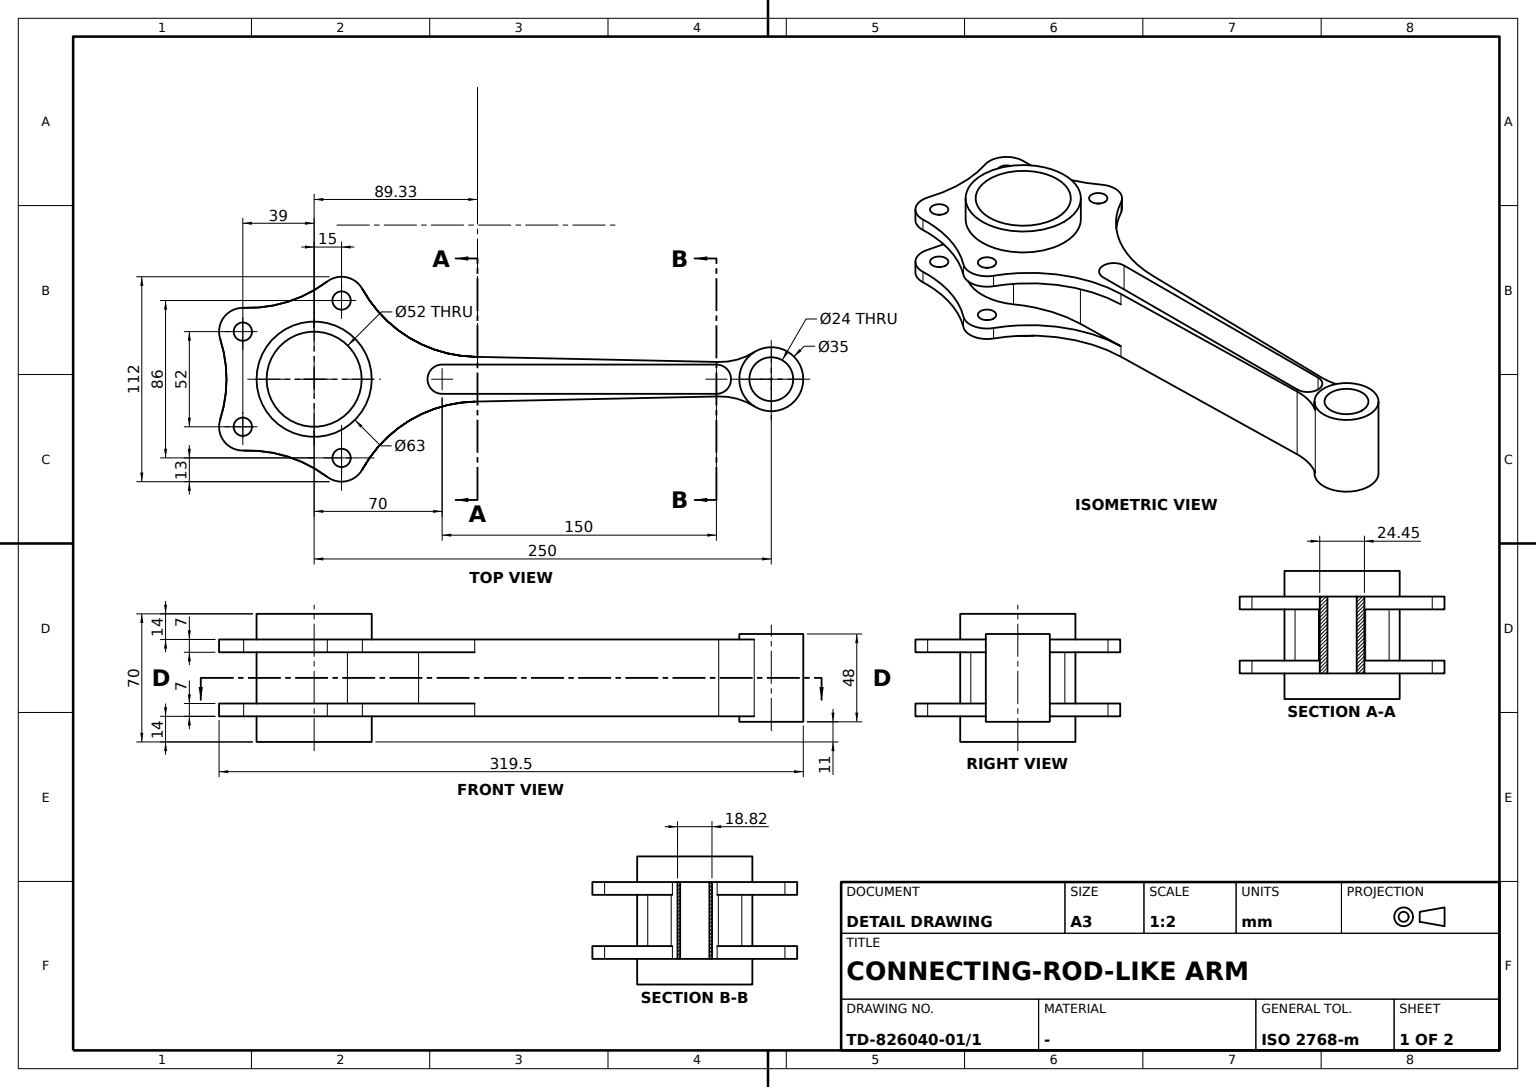
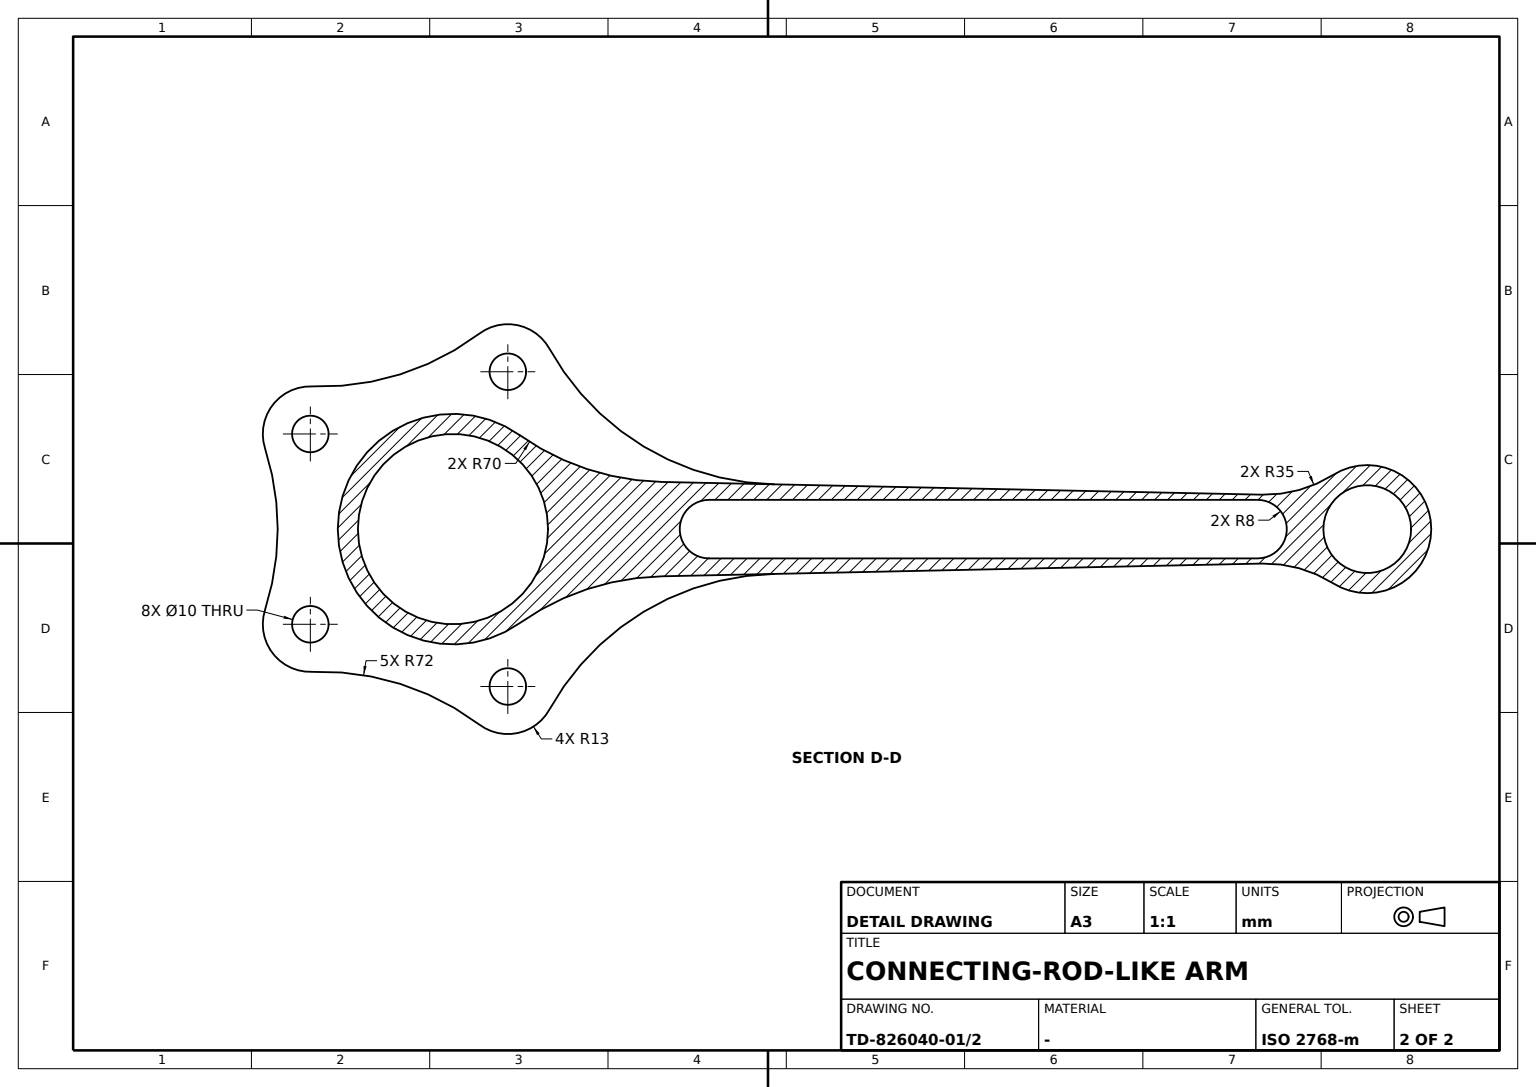
CATIA V5 part; units mm, degrees
sketch "Sketch1" plane through (0, 0, 0) normal (0, 0, 1) x (1, 0, 0)
  circle A0 centre (0, 0) radius 31.5
  circle A1 centre (0, 0) radius 26
  dimension "radius A1" = 26
  dimension "radius A0" = 31.5
extrude "Pad1" add sketch "Sketch1" along normal mid plane 70
sketch "Sketch2" plane through (0, 0, 0) normal (0, 0, 1) x (1, 0, 0)
  arc A0 (18.1862, -25.7199) -> (18.1862, 25.7199) centre (0, 0) ccw
  arc A1 (240.6635, 14.8014) -> (240.6635, -14.8014) centre (250, 0) ccw
  point P0 (250, 0)
  line L0 (70, 0) -> (220, 0) construction
  point P1 (70, 0)
  point P2 (220, 0)
  line L1 (70, 8) -> (220, 8)
  line L2 (220, -8) -> (70, -8)
  arc A2 (220, 8) -> (220, -8) centre (220, 0) cw
  arc A3 (70, -8) -> (70, 8) centre (70, 0) cw
  line L3 (57.1166, 12.8909) -> (221.2489, 9.4119)
  point P3 (75.5589, 12.5)
  point P4 (217.0947, 9.5)
  arc A4 (18.1862, 25.7199) -> (57.1166, 12.8909) centre (58.5999, 82.8752) ccw
  point P5 (18.1862, 25.7199)
  point P6 (57.1166, 12.8909)
  arc A5 (240.6635, 14.8014) -> (221.2489, 9.4119) centre (221.9906, 44.4041) cw
  point P7 (240.6635, 14.8014)
  point P8 (221.2489, 9.4119)
  point P9 (57.1166, -12.8909)
  point P10 (18.1862, -25.7199)
  arc A6 (18.1862, -25.7199) -> (57.1166, -12.8909) centre (58.5999, -82.8752) cw
  point P11 (221.2489, -9.4119)
  point P12 (57.1166, -12.8909)
  line L4 (57.1166, -12.8909) -> (221.2489, -9.4119)
  point P13 (221.2489, -9.4119)
  point P14 (240.6635, -14.8014)
  arc A7 (240.6635, -14.8014) -> (221.2489, -9.4119) centre (221.9906, -44.4041) ccw
  dimension "radius A0" = 31.5
  dimension "radius A1" = 17.5
  dimension "distance origin P0" = 250
  dimension "distance L0 L1" = 8
  dimension "distance P0 P2" = 30
  dimension "length L0" = 150
  dimension "distance P3 L0" = 12.5
  dimension "distance P4 L0" = 9.5
  dimension "radius A4" = 70
  dimension "radius A5" = 35
  constraint coincidence P0 x-axis
  constraint coincidence P1 x-axis
  constraint coincidence L3 P3
  constraint coincidence L3 P4
  constraint coincidence P9 P12
  constraint coincidence P11 P13
  constraint horizontal L0 x-axis
  constraint tangency A2 L1
  constraint tangency A3 L1
  constraint tangency A2 L2
  constraint tangency A3 L2
  constraint tangency A4 A0
  constraint tangency A4 L3
  constraint tangency A5 L3
  constraint tangency A5 A1
  constraint symmetry P6 P9 L0
  constraint symmetry P5 P10 L0
  constraint symmetry A4 A6 L0
  constraint symmetry P8 P11 L0
  constraint symmetry P6 P12 L0
  constraint symmetry L3 L4 L0
  constraint symmetry P8 P13 L0
  constraint symmetry P7 P14 L0
  constraint symmetry A5 A7 L0
extrude "Pad2" add sketch "Sketch2" along normal mid plane 42
sketch "Sketch3" plane through (0, 0, 21) normal (0, 0, 1) x (1, 0, 0)
  circle A0 centre (0, 0) radius 31.5
  arc A1 (-38.5515, 38.9923) -> (-51.3769, 22.0235) centre (-39, 26) ccw
  point P0 (-39, 26)
  circle A2 centre (-39, 26) radius 5
  arc A3 (26.3688, 49.3049) -> (7.1897, 53.3923) centre (15, 43) ccw
  point P1 (15, 43)
  circle A4 centre (15, 43) radius 5
  arc A5 (-38.5515, -38.9923) -> (-51.3769, -22.0235) centre (-39, -26) cw
  circle A6 centre (-39, -26) radius 5
  circle A7 centre (15, -43) radius 5
  arc A8 (26.3688, -49.3049) -> (7.1897, -53.3923) centre (15, -43) cw
  arc A9 (-38.5515, 38.9923) -> (7.1897, 53.3923) centre (-36.0674, 110.9494) ccw
  arc A10 (-51.3769, 22.0235) -> (-51.3769, -22.0235) centre (-119.9259, 0) cw
  arc A11 (-38.5515, -38.9923) -> (7.1897, -53.3923) centre (-36.0674, -110.9494) cw
  arc A12 (26.3688, 49.3049) -> (87.8084, 12.2404) centre (89.3342, 84.2242) ccw
  point P2 (26.3688, 49.3049)
  point P3 (87.8084, 12.2404)
  point P4 (87.8084, -12.2404)
  point P5 (26.3688, -49.3049)
  arc A13 (26.3688, -49.3049) -> (87.8084, -12.2404) centre (89.3342, -84.2242) cw
  line L0 (87.8084, 12.2404) -> (87.8084, -12.2404)
  dimension "radius A0" = 31.5
  dimension "radius A2" = 5
  dimension "radius A1" = 13
  dimension "radius A4" = 5
  dimension "radius A3" = 13
  dimension "distance y axis P0" = 39
  dimension "distance P0 x axis" = 26
  dimension "distance P1 y axis" = 15
  dimension "distance P0 P1 y axis" = 17
  dimension "radius A9" = 72
  dimension "radius A10" = 72
  dimension "radius A11" = 72
  dimension "radius A12" = 72
  constraint symmetry A1 A5 x-axis
  constraint symmetry A2 A6 x-axis
  constraint symmetry A4 A7 x-axis
  constraint symmetry A3 A8 x-axis
  constraint symmetry P3 P4 x-axis
  constraint symmetry P2 P5 x-axis
  constraint symmetry A12 A13 x-axis
  constraint tangency A9 A1
  constraint tangency A9 A3
  constraint tangency A10 A1
  constraint tangency A10 A5
  constraint tangency A11 A5
  constraint tangency A11 A8
  constraint tangency A12 A3
  constraint vertical L0 y-axis
extrude "Pad3" add sketch "Sketch3" against normal blind 7
mirror "Mirror1" about plane through (0, 0, 0) normal (0, 0, 1)
sketch "Sketch4" plane through (0, 0, 0) normal (0, 0, 1) x (1, 0, 0)
  arc A0 (220, -8) -> (220, 8) centre (220, 0) ccw
  line L0 (220, 8) -> (87.8084, 8)
  line L1 (87.8084, -8) -> (220, -8)
  line L2 (70, 8) -> (87.8084, 8)
  arc A1 (70, 8) -> (70, -8) centre (70, 0) ccw
  line L3 (70, -8) -> (87.8084, -8)
extrude "Pocket1" cut sketch "Sketch4" against normal through all and the other way through all
sketch "Sketch6" plane through (0, 0, 0) normal (0, 0, 1) x (1, 0, 0)
  circle A0 centre (250, 0) radius 12
  point P0 (250, 0)
  circle A1 centre (250, 0) radius 17.5
  dimension "radius A1" = 17.5
  dimension "radius A0" = 12
  dimension "distance y axis P0" = 250
  constraint coincidence P0 x-axis
extrude "Pad4" add sketch "Sketch6" along normal mid plane 48
sketch "Sketch5" plane through (0, 0, 0) normal (0, 1, 0) x (-1, 0, 0)
  point P0 (-124.0646, 12)
  point P1 (-85.5265, 21)
